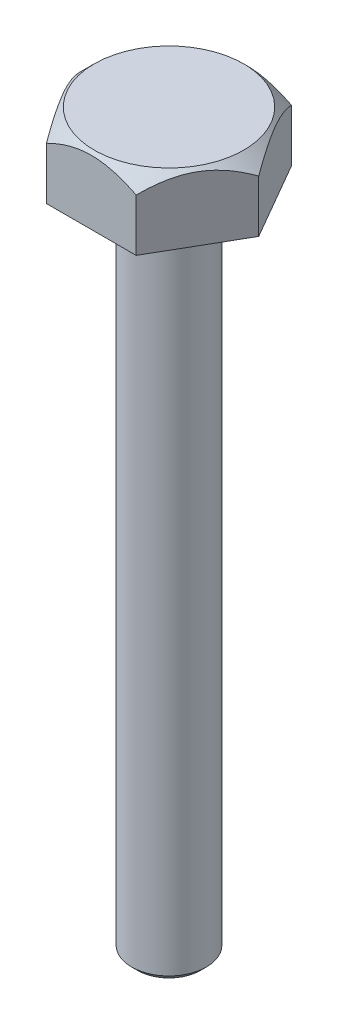
SolidWorks part; units mm, degrees
material "Zinc Alloy 7; AG40B; Zn-4Al-0.015Mg"
ref_plane "Front Plane" through (0, 0, 0) normal (0, 0, 1) x (1, 0, 0)
ref_plane "Top Plane" through (0, 0, 0) normal (0, 1, 0) x (1, 0, 0)
ref_plane "Right Plane" through (0, 0, 0) normal (1, 0, 0) x (0, 0, -1)
sketch "Hex Head Sketch AF104" plane through (0, 0, 0) normal (0, 1, 0) x (1, 0, 0)
  line L1 (60.0444, 0) -> (30.0222, 52)
  line L2 (30.0222, 52) -> (-30.0222, 52)
  line L3 (-30.0222, 52) -> (-60.0444, 0)
  line L4 (-60.0444, 0) -> (-30.0222, -52)
  line L5 (-30.0222, -52) -> (30.0222, -52)
  line L6 (30.0222, -52) -> (60.0444, 0)
  circle A0 centre (0, 0) radius 52 construction
  dimension "D1" = 104
extrude "Hex Head" add sketch "Hex Head Sketch AF104" against normal blind 45
sketch "Head Chamfer Profile" plane through (0, 0, 0) normal (0, 0, 1) x (1, 0, 0)
  line L0 (50.0444, 0) -> (60.0444, 0)
  line L1 (60.0444, 0) -> (60.0444, -10)
  line L2 (60.0444, -10) -> (50.0444, 0)
  line L3 (0, 0) -> (0, -45) construction
  line L4 (-30.0222, -45) -> (30.0222, -45) construction
  dimension "D1" = 10
  dimension "D2" = 10
revolve "Head Corner Chamfer Cut" cut sketch "Head Chamfer Profile" angle 360 about L3
sketch "Shank Sketch Ø50" plane through (0, 0, 0) normal (0, 1, 0) x (1, 0, 0)
  circle A0 centre (0, 0) radius 25
  dimension "D1" = 50
extrude "Shank Ø50x490" add sketch "Shank Sketch Ø50" against normal blind 490
chamfer "Shank End Chamfer 4x45°" distance 4 angle 45 1 edges at (0, -490, 25)
